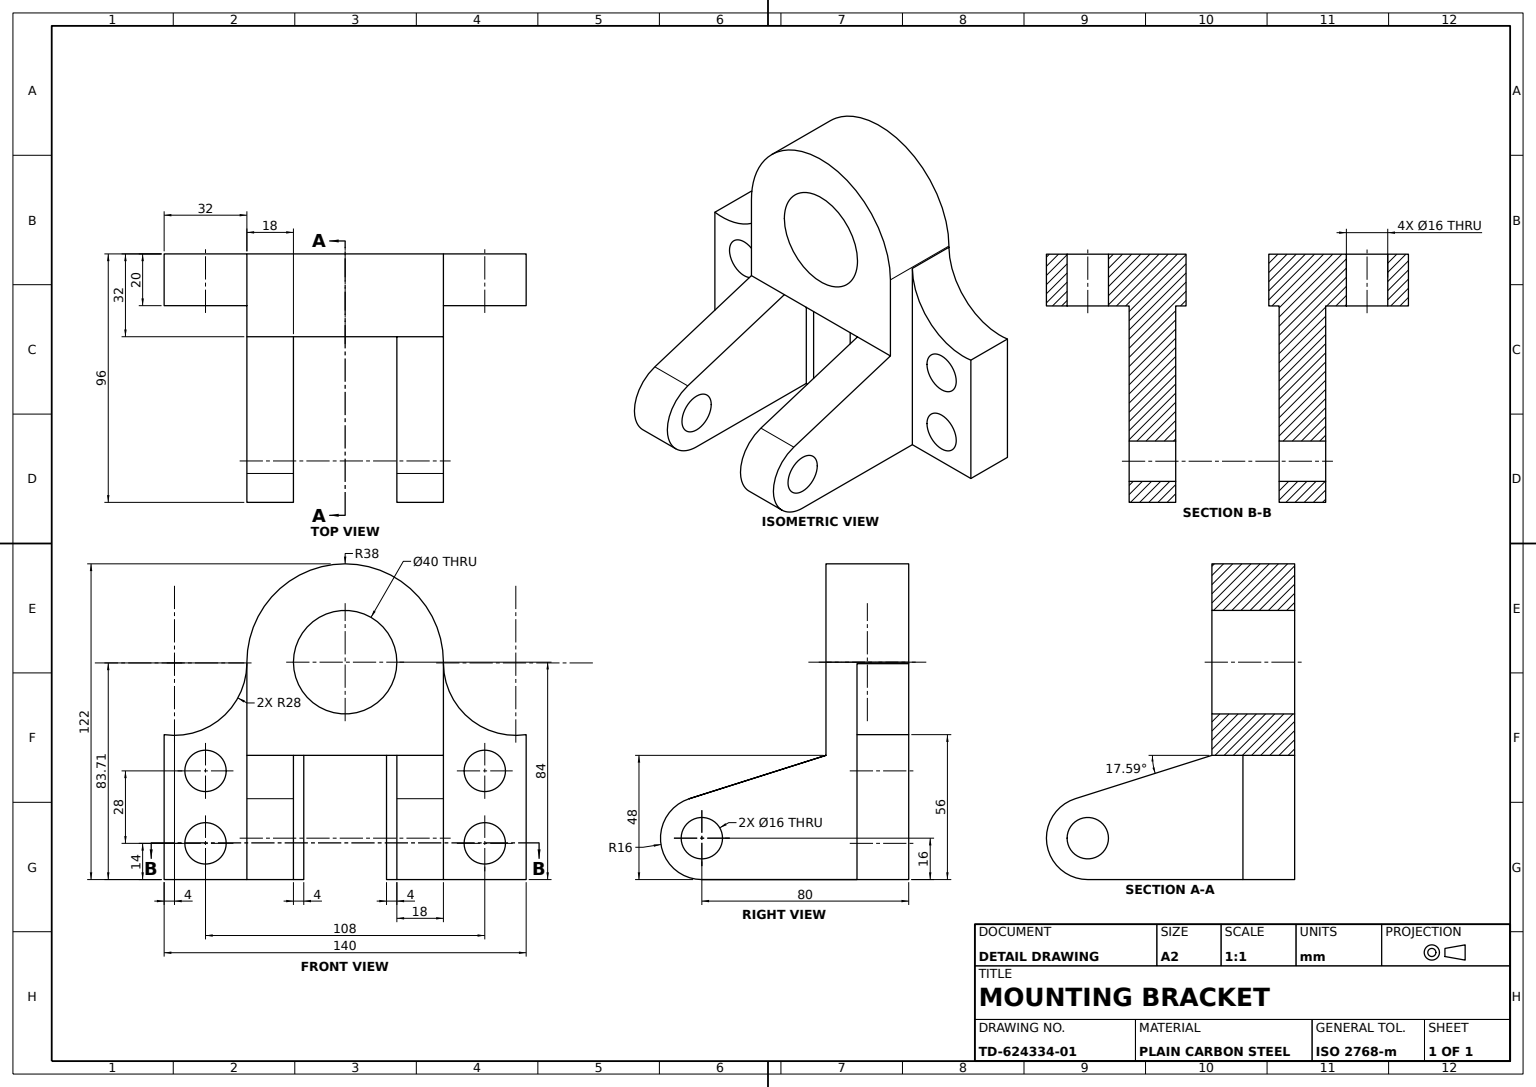
SolidWorks part; units mm, degrees
material "Plain Carbon Steel"
ref_plane "Front Plane" through (0, 0, 0) normal (0, 0, 1) x (1, 0, 0)
ref_plane "Top Plane" through (0, 0, 0) normal (0, 1, 0) x (1, 0, 0)
ref_plane "Right Plane" through (0, 0, 0) normal (1, 0, 0) x (0, 0, -1)
sketch "Hub Profile Sketch" plane through (0, 0, 0) normal (1, 0, 0) x (0, 0, -1)
  line L0 (-38, 0) -> (-38, -36)
  line L1 (-38, -36) -> (38, -36)
  line L2 (38, -36) -> (38, 0)
  circle A0 centre (0, 0) radius 20
  arc A1 (38, 0) -> (-38, 0) centre (0, 0) ccw
  dimension "D1" = 40
  dimension "D2" = 38
  dimension "D3" = 36
extrude "Hub Boss" add sketch "Hub Profile Sketch" along normal mid plane 32
sketch "Arm Profile Sketch" plane through (0, 0, 38) normal (0, 0, 1) x (1, 0, 0)
  line L0 (-16, -36) -> (-16, -84)
  line L1 (-16, -84) -> (64, -84)
  line L2 (16, -36) -> (68.8347, -52.7479)
  line L4 (-16, 0) -> (-16, -36)
  line L5 (-16, -36) -> (16, -36)
  line L6 (16, -36) -> (16, 0)
  line L7 (16, 0) -> (-16, 0)
  line L8 (-16, 0) -> (-16, -36)
  line L9 (-16, -36) -> (16, -36)
  line L10 (16, -36) -> (16, 0)
  line L11 (16, 0) -> (-16, 0)
  circle A0 centre (64, -68) radius 8
  arc A1 (68.8347, -52.7479) -> (64, -84) centre (64, -68) cw
  line M10 (-16, -36) -> (16, -36)
  dimension "D2" = 16
  dimension "D3" = 16
  dimension "D4" = 48
  dimension "D5" = 80
  dimension "D1" = 0
extrude "Arm Boss" add sketch "Arm Profile Sketch" against normal blind 18 contours A1 L2 L0 L1 A0 M10
mirror "Arm Mirror" about plane through (0, 0, 0) normal (0, 0, 1) of "Arm Boss"
sketch "Flange Profile Sketch" plane through (-16, 0, 0) normal (-1, 0, 0) x (0, 0, 1)
  line L0 (38, 0) -> (38, -84) construction
  line L1 (38, 0) -> (38, -84)
  line L2 (38, -84) -> (70, -84)
  line L3 (70, -84) -> (70, -28)
  arc A0 (38, 0) -> (70, -28) centre (65.9985, -0.2874) ccw
  circle A1 centre (54, -42) radius 8
  circle A2 centre (54, -70) radius 8
  line M14 (38, -84) -> (38, 0)
  dimension "D3" = 28
  dimension "D4" = 16
  dimension "D5" = 28
  dimension "D1" = 32
  dimension "D2" = 56
  dimension "D6" = 16
  dimension "D7" = 14
extrude "Flange Boss" add sketch "Flange Profile Sketch" against normal blind 20 contours A0 L2 L3 A2 A1 M14
mirror "Flange Mirror" about plane through (0, 0, 0) normal (0, 0, 1) of "Flange Boss"
sketch "Web Profile Sketch" plane through (-16, 0, 0) normal (-1, 0, 0) x (0, 0, 1)
  line L0 (-20, -84) -> (-16, -84)
  line L1 (-16, -84) -> (-16, -36)
  line L9 (-38, 0) -> (-38, -0.5748)
  line L10 (-70, -28) -> (-70, -84)
  line L11 (-70, -84) -> (-20, -84)
  line L12 (-20, -84) -> (-20, -36)
  line L13 (-20, -36) -> (20, -36)
  line L14 (20, -36) -> (20, -84)
  line L15 (20, -84) -> (70, -84)
  line L16 (70, -84) -> (70, -28)
  line L17 (38, -0.5748) -> (38, 0)
  line L18 (-38, 0) -> (-38, -0.5748)
  line L19 (-70, -28) -> (-70, -84)
  line L20 (-70, -84) -> (-20, -84)
  line L21 (-20, -84) -> (-20, -36)
  line L22 (-20, -36) -> (20, -36)
  line L23 (20, -36) -> (20, -84)
  line L24 (20, -84) -> (70, -84)
  line L25 (70, -84) -> (70, -28)
  line L26 (38, -0.5748) -> (38, 0)
  arc A3 (38, 0) -> (-38, 0) centre (0, 0) ccw
  arc A4 (-70, -28) -> (-38, -0.5748) centre (-65.9985, -0.2874) ccw
  arc A5 (38, -0.5748) -> (70, -28) centre (65.9985, -0.2874) ccw
  arc A6 (38, 0) -> (-38, 0) centre (0, 0) ccw
  arc A7 (-70, -28) -> (-38, -0.5748) centre (-65.9985, -0.2874) ccw
  arc A8 (38, -0.5748) -> (70, -28) centre (65.9985, -0.2874) ccw
  line M19 (-20, -84) -> (-20, -36)
  line M20 (-20, -36) -> (20, -36)
  dimension "D2" = 4
  dimension "D1" = 0
extrude "Web Boss" add sketch "Web Profile Sketch" against normal blind 20 contours L0 L1 M20 M19
mirror "Web Mirror" about plane through (0, 0, 0) normal (0, 0, 1) of "Web Boss"
